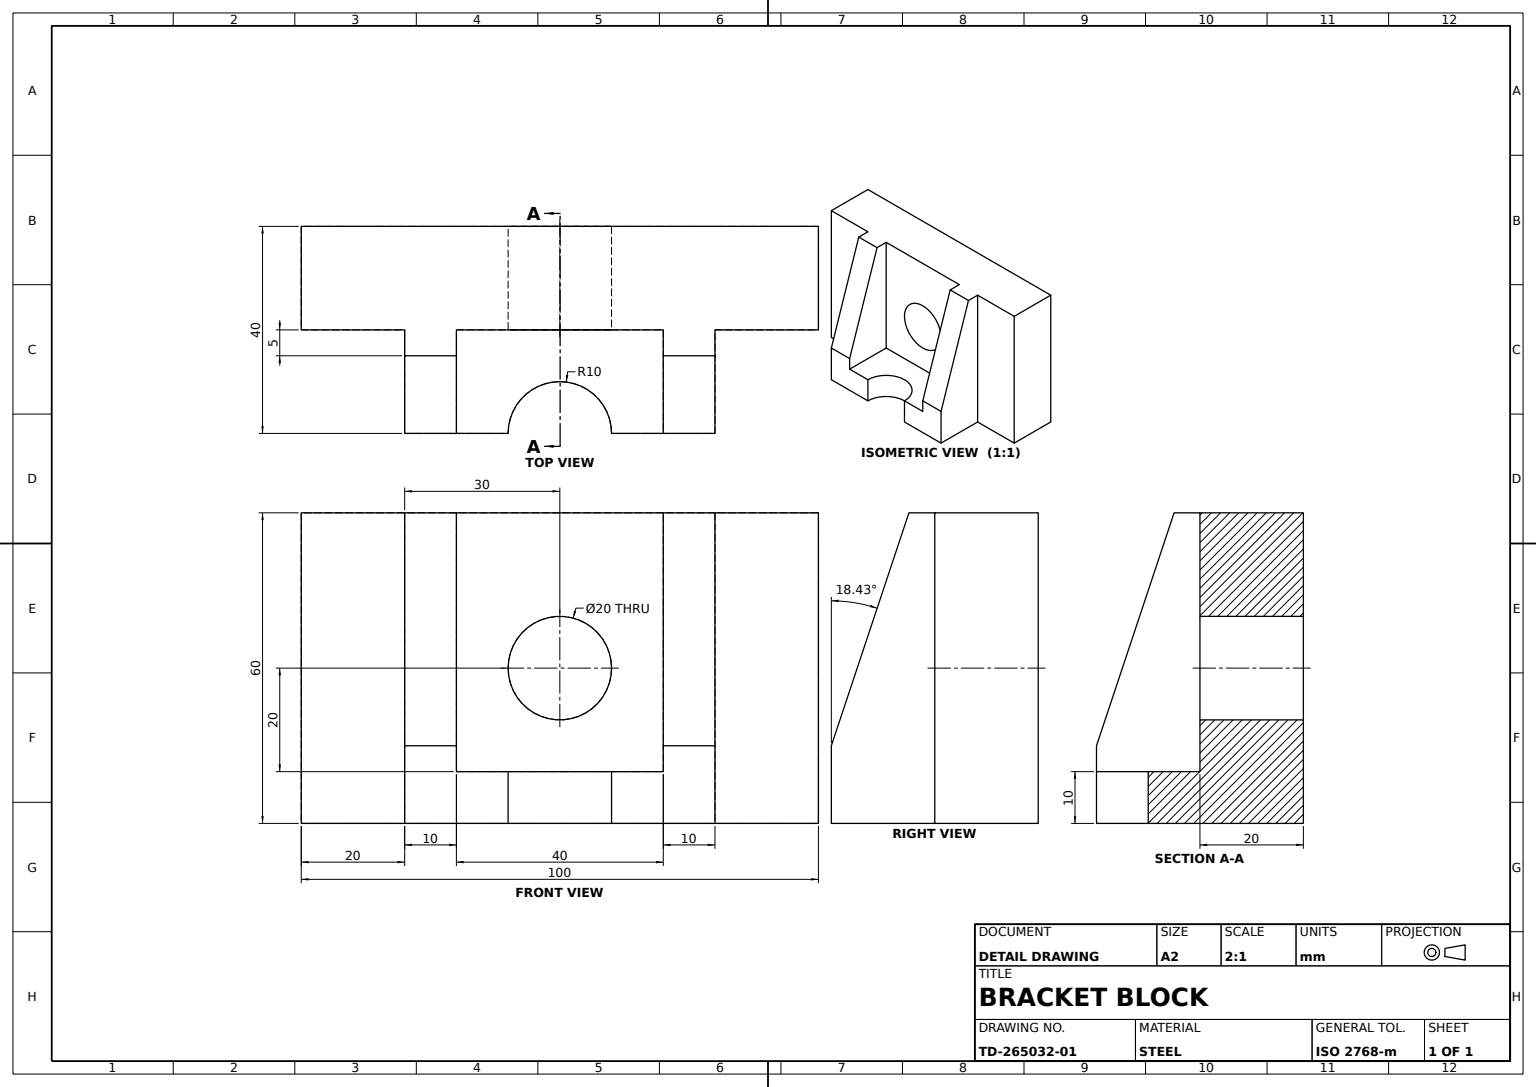
from build123d import *

# Parameters (mm, degrees)
BACK_PLATE_SKETCH_W       = 100
BACK_PLATE_SKETCH_H       = 60
BACK_PLATE_DEPTH          = 20
BORE_20_SKETCH_R          = 10
BORE_20_DEPTH             = 20
NOTCHED_BASE_FLANGE_DEPTH = 10
LEFT_GUSSET_DEPTH         = 10
RIGHT_GUSSET_DEPTH        = 10


with BuildPart() as part:
    # Back Plate Sketch → Back Plate (new body)
    with BuildSketch(Plane.XY):
        with Locations((50, 30)):
            Rectangle(BACK_PLATE_SKETCH_W, BACK_PLATE_SKETCH_H)
    extrude(amount=BACK_PLATE_DEPTH)

    # Bore Ø20 Sketch → Bore Ø20 (cut)
    with BuildSketch(Plane.XY.offset(20)):
        with Locations((50, 30)):
            Circle(BORE_20_SKETCH_R)
    extrude(amount=-BORE_20_DEPTH, mode=Mode.SUBTRACT)

    # Base Flange Sketch → Notched Base Flange (add)
    with BuildSketch(Plane.XZ):
        with BuildLine():
            Line((20, 20), (20, 40))
            Line((20, 40), (40, 40))
            ThreePointArc((40, 40), (50, 30), (60, 40))
            Line((60, 40), (80, 40))
            Line((80, 40), (80, 20))
            Line((80, 20), (20, 20))
        make_face()
    extrude(amount=-NOTCHED_BASE_FLANGE_DEPTH)

    # Left Gusset Sketch → Left Gusset (add)
    with BuildSketch(Plane(origin=(80, 0, 0), x_dir=(0, 0, -1), z_dir=(1, 0, 0))):
        Polygon((-40, 10), (-40, 15), (-25, 60), (-20, 60), (-20, 10), align=None)
    extrude(amount=-LEFT_GUSSET_DEPTH)

    # Right Gusset Sketch → Right Gusset (add)
    with BuildSketch(Plane.ZY.offset(-20)):
        Polygon((40, 10), (40, 15), (25, 60), (20, 60), (20, 10), align=None)
    extrude(amount=-RIGHT_GUSSET_DEPTH)


solid = part.part
